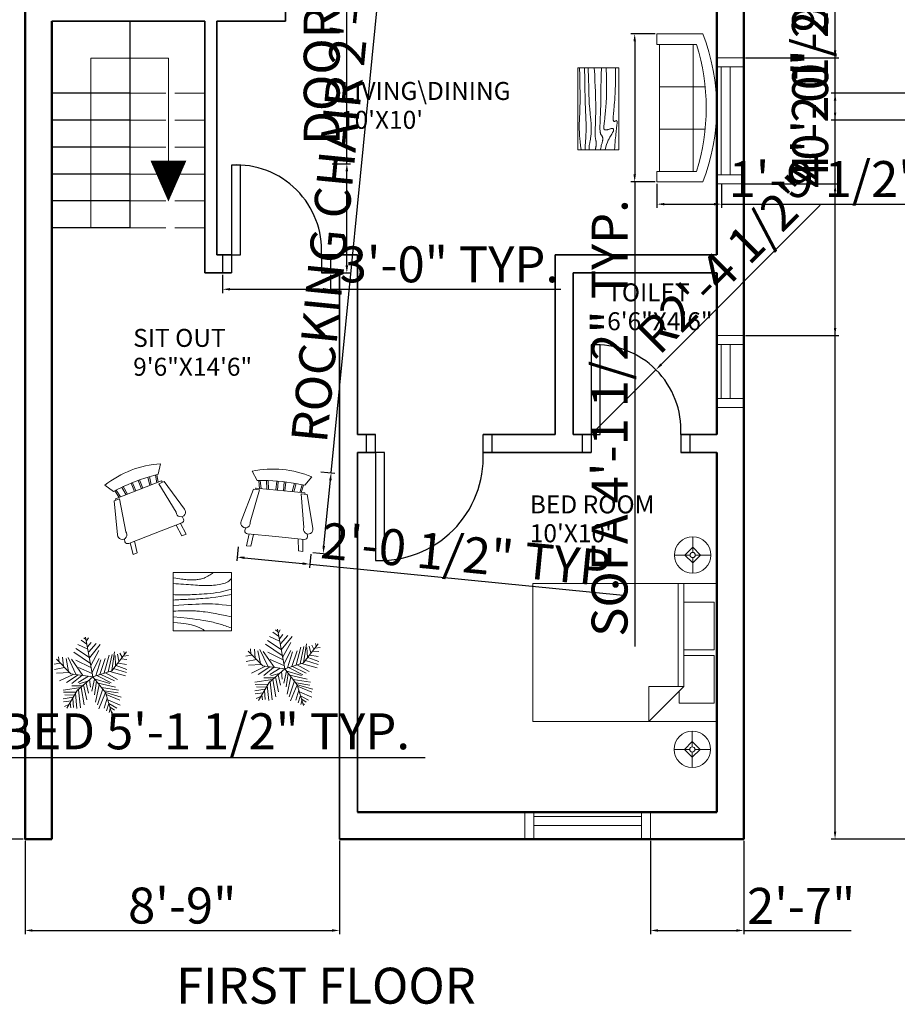
# Model space of a CAD drawing. Units: inches. Extents: x 2296 to 3335, y 495 to 1294.
# Tile 2 of 7: x 2659 to 2952, y 533 to 862. Entities that reach past the tile are written whole.
import ezdxf

# ---------------------------------------------------------------- set-up
doc = ezdxf.new("R2010")
doc.units = ezdxf.units.IN
doc.linetypes.add('ACAD_ISO02W100', pattern=[15, 12, -3])
for name, color, linetype, lineweight in [('A-ANNO-DIMS', 2, 'Continuous', 18), ('A-ANNO-SYMB', 7, 'Continuous', 18), ('A-ANNO-TEXT', 7, 'Continuous', 35), ('A-AREA-IDEN', 7, 'Continuous', 18), ('A-FLOR-STRS', 7, 'Continuous', 25), ('A-FLOR-STRS-OVHD', 7, 'ACAD_ISO02W100', 18), ('DOORS', 1, 'Continuous', 25), ('E-LITE', 2, 'Continuous', 18), ('FURNITURE', 2, 'Continuous', 18), ('INNER WALL', 6, 'Continuous', 35), ('L-PLNT', 3, 'Continuous', 13), ('OUTER WALL', 5, 'Continuous', 50), ('VENTILATOR', 4, 'Continuous', 18), ('WINDOWS', 3, 'Continuous', 18)]:
    doc.layers.add(name, color=color, linetype=linetype, lineweight=lineweight)
doc.styles.get("Standard").update_dxf_attribs({"font": 'arial.ttf'})
doc.dimstyles.new('ISO-25', dxfattribs={"dimtxt": 12, "dimasz": 2.5, "dimexe": 1.25, "dimexo": 0.625, "dimtad": 1, "dimdec": 1, "dimlunit": 3, "dimtxsty": 'Standard', "dimcen": 2.5, "dimadec": 0, "dimazin": 0, "dimtfac": 1, "dimtdec": 1, "dimtmove": 0, "dimatfit": 3, "dimfxl": 1, "dimarcsym": 0})

# ---------------------------------------------------------------- blocks, each defined once
blk = doc.blocks.new('Chair - Rocking')
for p, q in [((-8, -4.5), (-10, -1.5)), ((8, -4.5), (10, -1.5)), ((-7.5, -4.5), (-7, -7)), ((-6.5, -7), (-7.02225, -4.43)), ((-4.5, -7), (-4.96674, -4.19951)), ((-4, -7), (-4.40532, -4.16272)), ((-1.5, -4.05012), (-1.5, -7)), ((-1, -7), (-1, -4.05012)), ((1, -7), (1, -4.04655)), ((1.5, -4.05012), (1.5, -7)), ((4, -7), (4.40187, -4.18694)), ((4.5, -7), (4.96761, -4.19437)), ((6.5, -7), (7, -4.4057)), ((7.5, -4.5), (7, -7)), ((-9, -7.5), (-12, -18.49999)), ((-7, -7.5), (-9, -7.5)), ((-9, -18.49999), (-7, -7.5)), ((-8.23428, -6.99939), (-8.3093, -7.47958)), ((-8.23041, -7), (8.23915, -7)), ((7, -7.5), (9, -7.5)), ((9, -18.49999), (7, -7.5)), ((8.31071, -7.48854), (8.23449, -7.00073)), ((9, -7.5), (12, -18.49999)), ((-10.36644, -20.64523), (-10.5, -21.49999)), ((-9, -22.49999), (-9.5, -26.49999)), ((0, -22.49999), (-9.5, -22.49999)), ((-8, -26.49999), (-7.5, -22.49999)), ((0, -22.49999), (9.5, -22.49999)), ((8, -26.49999), (7.5, -22.49999)), ((9, -22.49999), (9.5, -26.49999)), ((10.5, -21.49999), (10.3575, -20.58798)), ((-9.5, -26.49999), (-8, -26.49999)), ((9.5, -26.49999), (8, -26.49999))]:
    blk.add_line(p, q)
for centre, radius, start, end in [((0, -34.08333), 34.08333, 72.93847, 107.0615), ((0, -68.25004), 64.25, 93.92211, 97.15267), ((0, -68.25004), 64.25, 82.84733, 93.92211), ((-10.5, -18.99999), 1.58114, 161.5651, 18.43495), ((10.5, -18.99999), 1.58114, 161.5651, 18.43495), ((-9.5, -21.49999), 1, 180, 270), ((9.5, -21.49999), 1, 270, 0)]:
    blk.add_arc(centre, radius, start, end)
blk = doc.blocks.new('Table - Square Woodgrain 42 x 42 in.')
blk.add_line((0, -42), (42, -42))
for points in [[(0, -4), (1.704, -4.2172), (3.2358, -4.4188), (4.615, -4.604), (5.8615, -4.7721), (6.9951, -4.9224), (8.0357, -5.0541), (9.0031, -5.1667), (9.9171, -5.2594), (10.7951, -5.3316), (11.6445, -5.3836), (12.4702, -5.4157), (13.277, -5.4283), (14.0698, -5.4217), (14.8535, -5.3964), (15.6331, -5.3526), (16.4133, -5.2908), (17.1986, -5.2103), (17.9913, -5.1062), (18.793, -4.9727), (19.6056, -4.8038), (20.4307, -4.5937), (21.2701, -4.3365), (22.1256, -4.0262), (22.9989, -3.6571), (23.888, -3.2272), (24.7756, -2.7516), (25.6408, -2.2491), (26.4624, -1.7387), (27.2195, -1.2395), (27.891, -0.7703), (28.456, -0.3501), (28.8934, 0.002)], [(0, -42), (0, 0), (42, 0), (42, -42)], [(0, -8), (1.8203, -8.1001), (3.6741, -8.2149), (5.5411, -8.3408), (7.4011, -8.4741), (9.2339, -8.6112), (11.0193, -8.7484), (12.7371, -8.8821), (14.3671, -9.0086), (15.8954, -9.1246), (17.3337, -9.2278), (18.6997, -9.3159), (20.0116, -9.387), (21.2871, -9.4389), (22.5442, -9.4696), (23.8008, -9.477), (25.0749, -9.459), (26.3791, -9.4137), (27.7049, -9.3403), (29.0383, -9.2382), (30.3655, -9.1068), (31.6728, -8.9455), (32.9461, -8.7535), (34.1717, -8.5304), (35.3358, -8.2756), (36.4268, -7.9863), (37.443, -7.6521), (38.3849, -7.2603), (39.253, -6.7986), (40.048, -6.2542), (40.7705, -5.6147), (41.421, -4.8674), (42, -4)], [(42, -12), (39.1784, -12.8621), (36.4519, -13.5654), (33.8246, -14.1294), (31.3004, -14.5731), (28.8832, -14.9161), (26.577, -15.1775), (24.3858, -15.3768), (22.3136, -15.5332), (20.3622, -15.6632), (18.5254, -15.7718), (16.7947, -15.8612), (15.1618, -15.9338), (13.6183, -15.9916), (12.1558, -16.0369), (10.7659, -16.0718), (9.4403, -16.0987), (8.1703, -16.1191), (6.9461, -16.1325), (5.7577, -16.1377), (4.595, -16.1335), (3.4479, -16.1188), (2.3064, -16.0924), (1.1604, -16.0532), (0, -16)], [(42, -16), (37.6529, -16.7365), (33.8802, -17.329), (30.6179, -17.7961), (27.8015, -18.1561), (25.3668, -18.4275), (23.2497, -18.6288), (21.3859, -18.7785), (19.7111, -18.8949), (18.1693, -18.9939), (16.7375, -19.0795), (15.401, -19.1534), (14.1449, -19.217), (12.9544, -19.2717), (11.8148, -19.3191), (10.7113, -19.3606), (9.6291, -19.3976), (8.5534, -19.4323), (7.47, -19.4689), (6.3643, -19.5122), (5.222, -19.5672), (4.0288, -19.6386), (2.7703, -19.7313), (1.4321, -19.8501), (0, -20)], [(0, -24), (3.9243, -23.6805), (7.4766, -23.4138), (10.6891, -23.1954), (13.5943, -23.0205), (16.2247, -22.8847), (18.6125, -22.7832), (20.7903, -22.7116), (22.7903, -22.6651), (24.6563, -22.642), (26.4764, -22.6507), (28.35, -22.7024), (30.3766, -22.8084), (32.6555, -22.98), (35.2861, -23.2283), (38.3678, -23.5645), (42, -24)], [(42, -32), (37.392, -31.017), (33.4585, -30.2231), (30.1291, -29.5949), (27.3334, -29.109), (25.0009, -28.742), (23.0612, -28.4707), (21.4439, -28.2716), (20.0786, -28.1215), (18.8998, -28.0002), (17.8609, -27.9014), (16.9206, -27.8219), (16.0371, -27.7588), (15.1691, -27.709), (14.2748, -27.6693), (13.3128, -27.6368), (12.2415, -27.6083), (11.0295, -27.5824), (9.6867, -27.5643), (8.233, -27.5608), (6.6884, -27.5787), (5.0728, -27.6248), (3.4062, -27.7058), (1.7086, -27.8286), (0, -28)], [(0, -32), (5.4026, -32.5358), (9.9494, -33.019), (13.7424, -33.4553), (16.8834, -33.8505), (19.4743, -34.2106), (21.6171, -34.5413), (23.4136, -34.8486), (24.9657, -35.1382), (26.3614, -35.4156), (27.6332, -35.6841), (28.7995, -35.9467), (29.8788, -36.2064), (30.8897, -36.4661), (31.8507, -36.7288), (32.7802, -36.9973), (33.6968, -37.2747), (34.6175, -37.5635), (35.5531, -37.8651), (36.5128, -38.1805), (37.506, -38.5108), (38.5421, -38.8568), (39.6302, -39.2197), (40.7797, -39.6004), (42, -40)], [(0, -36), (3.0098, -36.2857), (5.5354, -36.5643), (7.6368, -36.8359), (9.374, -37.1009), (10.807, -37.3597), (11.9957, -37.6126), (13.0002, -37.8599), (13.8804, -38.102), (14.6874, -38.3393), (15.4365, -38.5729), (16.1338, -38.8041), (16.7858, -39.0341), (17.3987, -39.264), (17.9787, -39.4952), (18.5322, -39.7288), (19.0655, -39.9662), (19.5832, -40.2081), (20.0842, -40.4544), (20.5657, -40.7046), (21.0249, -40.9581), (21.459, -41.2144), (21.8653, -41.4731), (22.2409, -41.7335), (22.5831, -41.9951)]]:
    blk.add_lwpolyline(points)
blk = doc.blocks.new('Sofa - Roundback 7 ft.')
for p, q in [((-12.00002, -32.4421), (-12.00003, -6.5971)), ((11.99997, -32.4421), (11.99998, -6.5971)), ((-36.000027, -34), (-36.000027, -11.4696)), ((-35.999844, -13.3819), (35.9998, -13.3819)), ((35.99998, -34), (35.99998, -11.4696)), ((-36.000027, -32.4421), (35.99998, -32.4421))]:
    blk.add_line(p, q)
for points in [[(-36.000027, -34), (-42.000027, -34), (-42.000027, -8)], [(41.99998, -8), (41.99998, -34), (35.99998, -34)]]:
    blk.add_lwpolyline(points)
for centre, radius, start, end in [((0, -114.25), 114.25, 68.43141, 111.5686), ((-0.00001, -127.1968), 121.1968, 72.72033, 107.2797)]:
    blk.add_arc(centre, radius, start, end)
blk = doc.blocks.new('Table - Rectangular Woodgrain 60 x 30 in.')
for p, q in [((0, 0), (0, -30)), ((60, 0), (0, 0)), ((60, -30), (60, 0)), ((0, -30), (60, -30))]:
    blk.add_line(p, q)
for points in [[(0, -2.4), (4.8155, -2.418), (9.0302, -2.4688), (12.709, -2.5477), (15.9167, -2.65), (18.7181, -2.7711), (21.1781, -2.9063), (23.3616, -3.0508), (25.3333, -3.2), (27.1477, -3.3495), (28.8172, -3.4958), (30.3437, -3.636), (31.7291, -3.7667), (32.9756, -3.8849), (34.0849, -3.9875), (35.059, -4.0714), (35.9, -4.1334), (36.6114, -4.1711), (37.2041, -4.1854), (37.6906, -4.1779), (38.0833, -4.15), (38.3948, -4.1034), (38.6375, -4.0396), (38.8239, -3.9602), (38.9666, -3.8667), (39.0764, -3.7608), (39.1573, -3.6448), (39.2116, -3.521), (39.2416, -3.3917), (39.2498, -3.2593), (39.2385, -3.1261), (39.21, -2.9944), (39.1666, -2.8667), (39.111, -2.7447), (39.0468, -2.6281), (38.978, -2.5163), (38.9083, -2.4083), (38.8418, -2.3035), (38.7823, -2.201), (38.7337, -2.1001), (38.7, -2), (38.6844, -1.9003), (38.6875, -1.8021), (38.7094, -1.707), (38.75, -1.6167), (38.8094, -1.5326), (38.8875, -1.4563), (38.9844, -1.3893), (39.1, -1.3333), (39.2351, -1.2896), (39.3937, -1.2583), (39.5804, -1.2396), (39.8, -1.2333), (40.057, -1.2396), (40.3562, -1.2583), (40.7023, -1.2896), (41.1, -1.3333), (41.5547, -1.3895), (42.0755, -1.4573), (42.6721, -1.5361), (43.3542, -1.625), (44.1316, -1.7233), (45.014, -1.8302), (46.0114, -1.9449), (47.1333, -2.0667), (48.3862, -2.1947), (49.7625, -2.3281), (51.2513, -2.4663), (52.8416, -2.6083), (54.5226, -2.7535), (56.2833, -2.9011), (58.1127, -3.0501), (60, -3.2)], [(0, -9.2), (6.5759, -9.0858), (11.9385, -9.0365), (16.2527, -9.0418), (19.6833, -9.0917), (22.3952, -9.1759), (24.5531, -9.2844), (26.322, -9.4069), (27.8666, -9.5333), (29.3241, -9.6553), (30.7203, -9.7719), (32.0532, -9.8837), (33.3208, -9.9917), (34.5213, -10.0965), (35.6526, -10.199), (36.7128, -10.2999), (37.7, -10.4), (38.6129, -10.4996), (39.4531, -10.5969), (40.223, -10.6895), (40.925, -10.775), (41.5613, -10.8512), (42.1344, -10.9156), (42.6465, -10.966), (43.1, -11), (43.4976, -11.0158), (43.8437, -11.0136), (44.143, -10.9942), (44.4, -10.9583), (44.6195, -10.9069), (44.8062, -10.8406), (44.9648, -10.7603), (45.1, -10.6667), (45.2155, -10.5598), (45.3114, -10.4365), (45.3871, -10.2929), (45.4416, -10.125), (45.4743, -9.929), (45.4844, -9.7011), (45.4709, -9.4371), (45.4333, -9.1333), (45.3716, -8.7883), (45.2896, -8.4104), (45.1919, -8.0107), (45.0833, -7.6), (44.9685, -7.1893), (44.8521, -6.7896), (44.7388, -6.4117), (44.6333, -6.0667), (44.54, -5.7628), (44.4614, -5.4979), (44.4001, -5.2675), (44.3583, -5.0667), (44.3384, -4.8909), (44.3427, -4.7354), (44.3736, -4.5956), (44.4333, -4.4667), (44.5236, -4.3453), (44.6427, -4.2333), (44.7884, -4.1339), (44.9583, -4.05), (45.1501, -3.9849), (45.3614, -3.9417), (45.59, -3.9234), (45.8333, -3.9333), (46.0915, -3.9749), (46.3734, -4.0531), (46.6906, -4.1736), (47.0542, -4.3417), (47.4756, -4.5629), (47.9661, -4.8427), (48.5372, -5.1866), (49.2, -5.6), (49.9676, -6.0844), (50.8594, -6.625), (51.8965, -7.2031), (53.1, -7.8), (54.491, -8.3969), (56.0906, -8.975), (57.9199, -9.5156), (60, -10)], [(0, -12.8), (5.1847, -12.9322), (9.6213, -13.0323), (13.3963, -13.1059), (16.5958, -13.1583), (19.3063, -13.1952), (21.614, -13.2219), (23.6054, -13.2439), (25.3666, -13.2667), (26.9728, -13.2947), (28.4531, -13.3281), (29.8256, -13.3663), (31.1083, -13.4083), (32.3191, -13.4535), (33.476, -13.501), (34.597, -13.5501), (35.7, -13.6), (36.7984, -13.6497), (37.8875, -13.6979), (38.9578, -13.743), (40, -13.7833), (41.0047, -13.8174), (41.9625, -13.8438), (42.864, -13.8607), (43.7, -13.8667), (44.4631, -13.8604), (45.1552, -13.8417), (45.7801, -13.8104), (46.3416, -13.7667), (46.8439, -13.7104), (47.2906, -13.6417), (47.6858, -13.5604), (48.0333, -13.4667), (48.3375, -13.3608), (48.6042, -13.2448), (48.8396, -13.121), (49.05, -12.9917), (49.2417, -12.8593), (49.4208, -12.7261), (49.5937, -12.5944), (49.7667, -12.4667), (49.9452, -12.3451), (50.1323, -12.2313), (50.3303, -12.1268), (50.5416, -12.0333), (50.7686, -11.9524), (51.0135, -11.8854), (51.2788, -11.8341), (51.5666, -11.8), (51.8785, -11.7843), (52.2116, -11.7865), (52.562, -11.8059), (52.926, -11.8417), (53.2998, -11.8931), (53.6795, -11.9594), (54.0614, -12.0397), (54.4416, -12.1333), (54.8223, -12.2401), (55.2293, -12.3625), (55.6942, -12.5037), (56.2489, -12.6667), (56.9251, -12.8547), (57.7545, -13.0708), (58.7689, -13.3182), (60, -13.6)], [(0, -18), (5.124, -17.7273), (9.6609, -17.5057), (13.6705, -17.3303), (17.2125, -17.1958), (20.3467, -17.0973), (23.1328, -17.0297), (25.6307, -16.9878), (27.9, -16.9667), (29.9928, -16.9617), (31.9302, -16.9703), (33.7254, -16.9907), (35.3917, -17.0208), (36.9423, -17.0588), (38.3906, -17.1026), (39.7499, -17.1503), (41.0333, -17.2), (42.2519, -17.2496), (43.4073, -17.2969), (44.4986, -17.3395), (45.525, -17.375), (46.4858, -17.4012), (47.3802, -17.4156), (48.2074, -17.416), (48.9667, -17.4), (49.6583, -17.3662), (50.2872, -17.3167), (50.8595, -17.2547), (51.3812, -17.1833), (51.8584, -17.1057), (52.2971, -17.025), (52.7034, -16.9443), (53.0833, -16.8667), (53.443, -16.7951), (53.789, -16.7313), (54.128, -16.6768), (54.4666, -16.6334), (54.8115, -16.6024), (55.1693, -16.5854), (55.5465, -16.5841), (55.95, -16.6), (56.3828, -16.6337), (56.8346, -16.6823), (57.2915, -16.7418), (57.7396, -16.8084), (58.165, -16.878), (58.5539, -16.9469), (58.8924, -17.0111), (59.1666, -17.0667), (59.3679, -17.1107), (59.5078, -17.1438), (59.6032, -17.1675), (59.6708, -17.1833), (59.7275, -17.193), (59.7901, -17.1979), (59.8753, -17.1998), (60, -17.2)], [(0, -22.4), (8.0098, -22.2501), (14.4094, -22.1011), (19.4168, -21.9535), (23.25, -21.8083), (26.1269, -21.6663), (28.2656, -21.5281), (29.884, -21.3947), (31.2, -21.2667), (32.3967, -21.1448), (33.5172, -21.0292), (34.5697, -20.9198), (35.5625, -20.8167), (36.5037, -20.7198), (37.4015, -20.6292), (38.2642, -20.5448), (39.1, -20.4667), (39.9164, -20.3951), (40.7187, -20.3313), (41.5117, -20.2768), (42.3, -20.2333), (43.0883, -20.2024), (43.8812, -20.1854), (44.6836, -20.1841), (45.5, -20.2), (46.3328, -20.234), (47.1747, -20.2844), (48.0163, -20.3488), (48.8479, -20.425), (49.66, -20.5106), (50.4429, -20.6031), (51.1872, -20.7004), (51.8833, -20.8), (52.5246, -20.8999), (53.1166, -20.9995), (53.6681, -21.0983), (54.1875, -21.1958), (54.6834, -21.2919), (55.1646, -21.3859), (55.6394, -21.4777), (56.1167, -21.5667), (56.6028, -21.6515), (57.0961, -21.7266), (57.5929, -21.7852), (58.0896, -21.8208), (58.5823, -21.8268), (59.0674, -21.7964), (59.5412, -21.723), (60, -21.6)], [(0, -25.2), (8.6355, -25.0504), (15.7026, -24.9031), (21.4049, -24.7606), (25.9458, -24.625), (29.529, -24.4988), (32.3578, -24.3844), (34.6359, -24.284), (36.5667, -24.2), (38.3213, -24.1341), (39.9417, -24.0854), (41.437, -24.0523), (42.8167, -24.0333), (44.0901, -24.0268), (45.2667, -24.0313), (46.3557, -24.0451), (47.3667, -24.0667), (48.309, -24.0947), (49.1928, -24.1287), (50.0284, -24.168), (50.826, -24.2125), (51.5959, -24.2617), (52.3483, -24.3151), (53.0935, -24.3725), (53.8417, -24.4334), (54.6009, -24.497), (55.3699, -24.561), (56.1454, -24.6226), (56.9239, -24.6792), (57.7021, -24.7279), (58.4764, -24.7662), (59.2435, -24.7911), (60, -24.8)], [(0, -28.8), (5.6867, -28.6681), (10.45, -28.5698), (14.407, -28.5012), (17.675, -28.4584), (20.3711, -28.4374), (22.6125, -28.4344), (24.5164, -28.4455), (26.2, -28.4667), (27.762, -28.4947), (29.2276, -28.5281), (30.6033, -28.5663), (31.8958, -28.6084), (33.1118, -28.6535), (34.2578, -28.7011), (35.3405, -28.7501), (36.3666, -28.8), (37.3443, -28.8497), (38.288, -28.8974), (39.2137, -28.9412), (40.1375, -28.9792), (41.0753, -29.0093), (42.0432, -29.0297), (43.0572, -29.0384), (44.1333, -29.0333), (45.2936, -29.0114), (46.5843, -28.9641), (48.0579, -28.8816), (49.7666, -28.7542), (51.7629, -28.5721), (54.0989, -28.3255), (56.8272, -28.0048), (60, -27.6)]]:
    blk.add_lwpolyline(points)
blk = doc.blocks.new('Bed - Queen')
for p, q in [((0, -80.00003), (0, 0)), ((0, 0), (59.99999, 0)), ((59.99999, 0), (59.99999, -80.00003)), ((7.99999, -1.2), (28.79998, -1.2)), ((7.99999, -14.4), (7.99999, -1.2)), ((28.79998, -1.2), (28.79998, -14.4)), ((31.19999, -1.2), (51.99999, -1.2)), ((31.19999, -14.4), (31.19999, -1.2)), ((51.99999, -1.2), (51.99999, -16.4)), ((0, -14.4), (44.8, -14.4)), ((44.8, -16.8), (0, -16.8)), ((59.99999, -29.6), (44.8, -14.4)), ((44.8, -14.4), (44.8, -29.6)), ((51.99999, -16.4), (46.79936, -16.4)), ((44.8, -29.6), (59.99999, -29.6)), ((59.99999, -80.00003), (0, -80.00003))]:
    blk.add_line(p, q)
blk = doc.blocks.new('Lamp - Table')
for p, q in [((0, 7), (0, 1)), ((-1, 0), (-7, 0)), ((0, 3), (-3, 0)), ((-3, 0), (0, -3)), ((3, 0), (0, 3)), ((0, -3), (3, 0)), ((1, 0), (7, 0)), ((0, -1), (0, -7))]:
    blk.add_line(p, q)
for radius in [7, 1]:
    blk.add_circle((0, 0), radius)
blk = doc.blocks.new('*U15')
for p, q in [((0, 0), (-10.5, 57)), ((-7.288, 39.707), (-21.778, 46.673)), ((-8.737, 47.138), (-17.069, 52.711)), ((-10.186, 53.64), (-13.084, 55.962)), ((-9.099, 51.782), (-6.563, 55.962)), ((-7.65, 43.423), (-2.578, 49.46)), ((-5.839, 35.992), (4.667, 48.067)), ((-5.114, 27.632), (10.463, 46.673)), ((-48.585, 21.131), (-49.309, 29.026)), ((-43.513, 28.561), (-42.427, 15.558)), ((-3.665, 19.273), (-27.574, 35.527)), ((-5.114, 28.097), (-24.676, 40.636)), ((-2.941, 16.486), (8.652, 37.85)), ((16.259, 5.805), (23.142, 31.348)), ((22.055, 7.198), (27.489, 32.277)), ((27, 9), (48, 36)), ((27.127, 9.056), (31.112, 35.992)), ((31.836, 30.883), (32.561, 16.486)), ((35.096, 32.741), (37.27, 22.524)), ((38.719, 34.134), (41.979, 28.561)), ((43.791, 29.954), (51.036, 30.883)), ((44.153, 36.456), (45.239, 32.741)), ((-47.498, 19.737), (-55.83, 18.344)), ((-31.5, 4.5), (-52.5, 25.5)), ((-38.442, 26.239), (-34.819, 7.663)), ((-35.544, 28.097), (-24.314, 3.947)), ((-14.533, 2.09), (-30.834, 25.31)), ((-24.314, 23.917), (-2.941, 13.7)), ((-1.129, 6.734), (9.014, 26.704)), ((3.942, 1.625), (11.187, 24.381)), ((10.101, 3.483), (17.708, 26.239)), ((33.285, 16.486), (48.862, 10.913)), ((36.183, 19.737), (48.137, 17.88)), ((40.53, 25.775), (48.862, 24.846)), ((-40.615, 13.7), (-55.105, 10.913)), ((-33.37, 6.269), (-52.207, 5.34)), ((-28.299, 3.483), (-47.86, -5.805)), ((-21.416, 3.018), (-38.079, -8.128)), ((0, 0), (-31.5, 4.5)), ((-15.982, 2.09), (-30.11, -9.521)), ((0, 0), (-22.5, -19.5)), ((-6.563, 1.161), (-21.416, -8.128)), ((-20.691, 13.7), (-1.129, 4.876)), ((0, 0), (27, 9)), ((0, 0), (18, -22.5)), ((6.478, 1.625), (26.04, -8.592)), ((11.187, 3.483), (30.749, -5.805)), ((18.07, 5.805), (35.096, -3.483)), ((24.229, 7.663), (46.688, 1.625)), ((29.662, 12.307), (48.137, 6.269)), ((-15.257, -12.772), (-30.11, -12.772)), ((-6.563, -5.805), (-19.967, -9.985)), ((-13.446, -11.378), (-8.737, -32.741)), ((-9.461, -8.592), (-6.201, -23.453)), ((-4.752, -3.483), (-3.665, -14.629)), ((2.493, -3.019), (-1.491, -20.202)), ((1.769, -2.555), (24.229, -9.521)), ((5.029, -6.27), (2.131, -25.775)), ((9.014, -11.378), (3.58, -35.992)), ((7.565, -9.056), (32.198, -14.629)), ((-17.431, -15.094), (-42.789, -18.809)), ((-24.314, -21.596), (-42.427, -22.06)), ((-26.849, -26.24), (-40.253, -25.775)), ((-22.5, -19.5), (-37.5, -45)), ((-25.038, -23.918), (-22.865, -45.281)), ((-20.691, -18.345), (-17.793, -44.352)), ((-17.069, -15.094), (-12.721, -40.172)), ((14.085, -16.951), (6.478, -40.172)), ((18.07, -22.524), (8.289, -45.745)), ((12.274, -15.094), (36.907, -18.809)), ((16.259, -19.738), (36.183, -22.989)), ((18, -22.5), (27, -52.5)), ((18.433, -22.524), (40.53, -29.026)), ((19.157, -25.311), (38.719, -33.206)), ((-28.299, -29.026), (-42.789, -31.348)), ((-30.834, -34.135), (-42.427, -35.528)), ((-34.457, -39.708), (-40.978, -42.494)), ((-32.646, -36.921), (-31.921, -44.352)), ((-29.023, -30.884), (-27.936, -43.887)), ((20.244, -30.419), (15.897, -44.816)), ((22.78, -37.85), (19.519, -48.532)), ((21.331, -32.741), (39.081, -40.636)), ((22.78, -38.314), (34.372, -44.816)), ((24.591, -45.745), (23.142, -50.854)), ((24.591, -43.423), (30.749, -47.603)), ((26.764, -49.925), (28.213, -50.854))]:
    blk.add_line(p, q)
blk = doc.blocks.new('DOOR-SINGLE-30IN')
for p, q in [((-3, 0), (-3, -6)), ((0, 0), (0, -6)), ((30, 0), (30, -6)), ((33, 0), (33, -6))]:
    blk.add_line(p, q)
blk.add_lwpolyline([(0, 0), (3, 0), (3, 30), (0, 30)], close=True)
blk.add_arc((1.5, 1.5), 28.54, 356.9872, 93.0128)
blk = doc.blocks.new('DOOR-SINGLE-36IN')
for p, q in [((0, 39), (-6, 39)), ((0, 36), (-6, 36)), ((0, 0), (-6, 0)), ((0, -3), (-6, -3))]:
    blk.add_line(p, q)
blk.add_lwpolyline([(0, 0), (36, 0), (36, 3), (0, 3)], close=True)
blk.add_arc((1.5, 1.5), 34.53, 357.5104, 92.4896)
blk = doc.blocks.new('WIN-36IN')
for p, q in [((0, 42), (9, 42)), ((0, 39), (9, 39)), ((1.5, 3), (1.5, 39)), ((4.5, 3), (4.5, 39)), ((9, 3), (0, 3)), ((9, 0), (0, 0))]:
    blk.add_line(p, q)
blk = doc.blocks.new('VENT-18IN')
for p, q in [((0, 24), (9, 24)), ((0, 21), (9, 21)), ((4.5, 21), (4.5, 3)), ((7.5, 21), (7.5, 3)), ((9, 3), (0, 3)), ((9, 0), (0, 0))]:
    blk.add_line(p, q)
blk = doc.blocks.new('*D27')
at = {"layer": 'A-ANNO-DIMS', "color": 0, "lineweight": -2, "transparency": 16777216}
for p, q in [((2524.66, 623.83), (2524.66, 613.99)), ((2586.06, 623.83), (2586.06, 613.99)), ((2527.16, 615.24), (2583.56, 615.24)), ((2586.06, 615.24), (2794.3, 615.24))]:
    blk.add_line(p, q, dxfattribs=at)
at = {"layer": 'A-ANNO-DIMS', "color": 0, "transparency": 16777216}
for points in [[(2527.16, 615.66), (2527.16, 614.82), (2524.66, 615.24)], [(2583.56, 615.66), (2583.56, 614.82), (2586.06, 615.24)]]:
    blk.add_solid(points, dxfattribs=at)
at = {"layer": 'Defpoints', "color": 0, "transparency": 16777216}
for p in [(2524.66, 624.45), (2586.06, 624.45), (2586.06, 615.24)]:
    blk.add_point(p, dxfattribs=at)
at = {"layer": 'A-ANNO-DIMS', "color": 0, "transparency": 16777216, "insert": (2691.43, 622.44), "char_height": 12, "attachment_point": 5}
blk.add_mtext('QUEEN BED 5\'-1 1/2" TYP.', dxfattribs=at)
blk = doc.blocks.new('*D37')
at = {"layer": 'A-ANNO-DIMS', "color": 0, "lineweight": -2, "transparency": 16777216}
for p, q in [((2768.12, 813.44), (2768.12, 998.74)), ((2763.28, 813.44), (2769.37, 813.44)), ((2768.12, 779.52), (2768.12, 810.94)), ((2763.28, 777.02), (2769.37, 777.02))]:
    blk.add_line(p, q, dxfattribs=at)
at = {"layer": 'A-ANNO-DIMS', "color": 0, "transparency": 16777216}
for points in [[(2767.7, 810.94), (2768.54, 810.94), (2768.12, 813.44)], [(2767.7, 779.52), (2768.54, 779.52), (2768.12, 777.02)]]:
    blk.add_solid(points, dxfattribs=at)
at = {"layer": 'Defpoints', "color": 0, "transparency": 16777216}
for p in [(2762.66, 813.44), (2768.12, 813.44), (2762.66, 777.02)]:
    blk.add_point(p, dxfattribs=at)
at = {"layer": 'A-ANNO-DIMS', "color": 0, "transparency": 16777216, "insert": (2761.28, 907.34), "char_height": 12, "attachment_point": 5, "rotation": 90}
blk.add_mtext('DOOR D1 3\'-0 1/2" TYP.', dxfattribs=at)
blk = doc.blocks.new('*D38')
at = {"layer": 'A-ANNO-DIMS', "color": 0, "lineweight": -2, "transparency": 16777216}
for p, q in [((2726.66, 776.39), (2726.66, 770.3)), ((2762.66, 776.39), (2762.66, 770.3)), ((2729.16, 771.55), (2760.16, 771.55)), ((2762.66, 771.55), (2839.55, 771.55))]:
    blk.add_line(p, q, dxfattribs=at)
at = {"layer": 'A-ANNO-DIMS', "color": 0, "transparency": 16777216}
for points in [[(2729.16, 771.97), (2729.16, 771.14), (2726.66, 771.55)], [(2760.16, 771.97), (2760.16, 771.14), (2762.66, 771.55)]]:
    blk.add_solid(points, dxfattribs=at)
at = {"layer": 'Defpoints', "color": 0, "transparency": 16777216}
for p in [(2726.66, 777.02), (2762.66, 777.02), (2762.66, 771.55)]:
    blk.add_point(p, dxfattribs=at)
at = {"layer": 'A-ANNO-DIMS', "color": 0, "transparency": 16777216, "insert": (2802.35, 778.31), "char_height": 12, "attachment_point": 5}
blk.add_mtext('3\'-0" TYP.', dxfattribs=at)
blk = doc.blocks.new('*D43')
at = {"layer": 'A-ANNO-DIMS', "color": 0, "lineweight": -2, "transparency": 16777216}
for p, q in [((2871.03, 856.78), (2862.99, 856.78)), ((2864.24, 854.28), (2864.24, 809.87)), ((2871.03, 807.37), (2862.99, 807.37)), ((2864.24, 807.37), (2864.24, 652.27))]:
    blk.add_line(p, q, dxfattribs=at)
at = {"layer": 'A-ANNO-DIMS', "color": 0, "transparency": 16777216}
for points in [[(2863.83, 854.28), (2864.66, 854.28), (2864.24, 856.78)], [(2863.83, 809.87), (2864.66, 809.87), (2864.24, 807.37)]]:
    blk.add_solid(points, dxfattribs=at)
at = {"layer": 'Defpoints', "color": 0, "transparency": 16777216}
for p in [(2871.66, 856.78), (2864.24, 807.37), (2871.66, 807.37)]:
    blk.add_point(p, dxfattribs=at)
at = {"layer": 'A-ANNO-DIMS', "color": 0, "transparency": 16777216, "insert": (2857.41, 728.57), "char_height": 12, "attachment_point": 5, "rotation": 90}
blk.add_mtext('SOFA 4\'-1 1/2" TYP.', dxfattribs=at)
blk = doc.blocks.new('*D44')
at = {"layer": 'A-ANNO-DIMS', "color": 0, "lineweight": -2, "transparency": 16777216}
for p, q in [((2871.66, 806.74), (2871.66, 798.71)), ((2893.23, 806.74), (2893.23, 798.71)), ((2874.16, 799.96), (2890.73, 799.96)), ((2893.23, 799.96), (2996.95, 799.96))]:
    blk.add_line(p, q, dxfattribs=at)
at = {"layer": 'A-ANNO-DIMS', "color": 0, "transparency": 16777216}
for points in [[(2874.16, 800.37), (2874.16, 799.54), (2871.66, 799.96)], [(2890.73, 800.37), (2890.73, 799.54), (2893.23, 799.96)]]:
    blk.add_solid(points, dxfattribs=at)
at = {"layer": 'Defpoints', "color": 0, "transparency": 16777216}
for p in [(2871.66, 807.37), (2893.23, 807.37), (2893.23, 799.96)]:
    blk.add_point(p, dxfattribs=at)
at = {"layer": 'A-ANNO-DIMS', "color": 0, "transparency": 16777216, "insert": (2946.34, 806.78), "char_height": 12, "attachment_point": 5}
blk.add_mtext('1\'-9 1/2" TYP.', dxfattribs=at)
blk = doc.blocks.new('*D47')
at = {"layer": 'A-ANNO-DIMS', "color": 0, "lineweight": -2, "transparency": 16777216}
for p, q in [((2762.87, 710.27), (2784.09, 925.21)), ((2759.46, 710.6), (2764.11, 710.14)), ((2760.46, 685.88), (2762.62, 707.78)), ((2756.81, 683.73), (2761.46, 683.27))]:
    blk.add_line(p, q, dxfattribs=at)
at = {"layer": 'A-ANNO-DIMS', "color": 0, "transparency": 16777216}
for points in [[(2762.21, 707.82), (2763.04, 707.74), (2762.87, 710.27)], [(2760.04, 685.93), (2760.87, 685.84), (2760.21, 683.4)]]:
    blk.add_solid(points, dxfattribs=at)
at = {"layer": 'Defpoints', "color": 0, "transparency": 16777216}
for p in [(2758.84, 710.66), (2762.87, 710.27), (2756.18, 683.79)]:
    blk.add_point(p, dxfattribs=at)
at = {"layer": 'A-ANNO-DIMS', "color": 0, "transparency": 16777216, "insert": (2766.79, 819.65), "char_height": 12, "attachment_point": 5, "rotation": 84.3621}
blk.add_mtext('ROCKING CHAIR 2\'-3" TYP.', dxfattribs=at)
blk = doc.blocks.new('*D48')
at = {"layer": 'A-ANNO-DIMS', "color": 0, "lineweight": -2, "transparency": 16777216}
for p, q in [((2731.81, 685.57), (2731.35, 680.92)), ((2733.96, 681.92), (2753.3, 680.01)), ((2756.12, 683.17), (2755.66, 678.52)), ((2755.79, 679.76), (2860.34, 669.44))]:
    blk.add_line(p, q, dxfattribs=at)
at = {"layer": 'A-ANNO-DIMS', "color": 0, "transparency": 16777216}
for points in [[(2734, 682.33), (2733.92, 681.5), (2731.47, 682.16)], [(2753.34, 680.42), (2753.26, 679.6), (2755.79, 679.76)]]:
    blk.add_solid(points, dxfattribs=at)
at = {"layer": 'Defpoints', "color": 0, "transparency": 16777216}
for p in [(2731.87, 686.2), (2756.18, 683.79), (2755.79, 679.76)]:
    blk.add_point(p, dxfattribs=at)
at = {"layer": 'A-ANNO-DIMS', "color": 0, "transparency": 16777216, "insert": (2809.98, 681.28), "char_height": 12, "attachment_point": 5, "rotation": 354.3621}
blk.add_mtext('2\'-0 1/2" TYP.', dxfattribs=at)
blk = doc.blocks.new('*D52')
at = {"layer": 'A-ANNO-DIMS', "color": 0, "lineweight": -2, "transparency": 16777216}
for p, q in [((2660.03, 1068.02), (2628.91, 1068.02)), ((2630.16, 590.52), (2630.16, 1065.52)), ((2660.03, 588.02), (2628.91, 588.02))]:
    blk.add_line(p, q, dxfattribs=at)
at = {"layer": 'A-ANNO-DIMS', "color": 0, "transparency": 16777216}
for points in [[(2629.74, 1065.52), (2630.57, 1065.52), (2630.16, 1068.02)], [(2629.74, 590.52), (2630.57, 590.52), (2630.16, 588.02)]]:
    blk.add_solid(points, dxfattribs=at)
at = {"layer": 'Defpoints', "color": 0, "transparency": 16777216}
for p in [(2630.16, 1068.02), (2660.66, 1068.02), (2660.66, 588.02)]:
    blk.add_point(p, dxfattribs=at)
at = {"layer": 'A-ANNO-DIMS', "color": 0, "transparency": 16777216, "insert": (2623.41, 828.02), "char_height": 12, "attachment_point": 5, "rotation": 90}
blk.add_mtext('40\'-0"', dxfattribs=at)
blk = doc.blocks.new('*D54')
at = {"layer": 'A-ANNO-DIMS', "color": 0, "lineweight": -2, "transparency": 16777216}
for p, q in [((2961.02, 1068.02), (2929.9, 1068.02)), ((2931.15, 590.52), (2931.15, 1065.52)), ((2961.02, 588.02), (2929.9, 588.02))]:
    blk.add_line(p, q, dxfattribs=at)
at = {"layer": 'A-ANNO-DIMS', "color": 0, "transparency": 16777216}
for points in [[(2930.73, 1065.52), (2931.56, 1065.52), (2931.15, 1068.02)], [(2930.73, 590.52), (2931.56, 590.52), (2931.15, 588.02)]]:
    blk.add_solid(points, dxfattribs=at)
at = {"layer": 'Defpoints', "color": 0, "transparency": 16777216}
for p in [(2931.15, 1068.02), (2961.65, 1068.02), (2961.65, 588.02)]:
    blk.add_point(p, dxfattribs=at)
at = {"layer": 'A-ANNO-DIMS', "color": 0, "transparency": 16777216, "insert": (2924.39, 828.02), "char_height": 12, "attachment_point": 5, "rotation": 90}
blk.add_mtext('40\'-0"', dxfattribs=at)
blk = doc.blocks.new('*D66')
at = {"layer": 'A-ANNO-DIMS', "color": 0, "lineweight": -2, "transparency": 16777216}
for p, q in [((2931.15, 837.02), (2931.15, 872.67)), ((2970.02, 837.02), (2929.9, 837.02)), ((2931.15, 830.52), (2931.15, 834.52)), ((2970.02, 828.02), (2929.9, 828.02))]:
    blk.add_line(p, q, dxfattribs=at)
at = {"layer": 'A-ANNO-DIMS', "color": 0, "transparency": 16777216}
for points in [[(2930.73, 834.52), (2931.56, 834.52), (2931.15, 837.02)], [(2930.73, 830.52), (2931.56, 830.52), (2931.15, 828.02)]]:
    blk.add_solid(points, dxfattribs=at)
at = {"layer": 'Defpoints', "color": 0, "transparency": 16777216}
for p in [(2931.15, 837.02), (2970.65, 837.02), (2970.65, 828.02)]:
    blk.add_point(p, dxfattribs=at)
at = {"layer": 'A-ANNO-DIMS', "color": 0, "transparency": 16777216, "insert": (2924.39, 856.09), "char_height": 12, "attachment_point": 5, "rotation": 90}
blk.add_mtext('0\'-9"', dxfattribs=at)
blk = doc.blocks.new('*D68')
at = {"layer": 'A-ANNO-DIMS', "color": 0, "lineweight": -2, "transparency": 16777216}
for p, q in [((2901.28, 948.82), (2932.41, 948.82)), ((2931.16, 851.25), (2931.16, 946.32)), ((2901.28, 848.75), (2932.41, 848.75))]:
    blk.add_line(p, q, dxfattribs=at)
at = {"layer": 'A-ANNO-DIMS', "color": 0, "transparency": 16777216}
for points in [[(2930.74, 946.32), (2931.57, 946.32), (2931.16, 948.82)], [(2930.74, 851.25), (2931.57, 851.25), (2931.16, 848.75)]]:
    blk.add_solid(points, dxfattribs=at)
at = {"layer": 'Defpoints', "color": 0, "transparency": 16777216}
for p in [(2900.66, 948.82), (2931.16, 948.82), (2900.66, 848.75)]:
    blk.add_point(p, dxfattribs=at)
at = {"layer": 'A-ANNO-DIMS', "color": 0, "transparency": 16777216, "insert": (2924.41, 898.79), "char_height": 12, "attachment_point": 5, "rotation": 90}
blk.add_mtext('8\'-4"', dxfattribs=at)
blk = doc.blocks.new('*D69')
at = {"layer": 'A-ANNO-DIMS', "color": 0, "lineweight": -2, "transparency": 16777216}
for p, q in [((2931.16, 806.75), (2931.16, 870.85)), ((2901.28, 806.75), (2932.41, 806.75)), ((2931.16, 758.61), (2931.16, 804.25)), ((2901.28, 756.11), (2932.41, 756.11))]:
    blk.add_line(p, q, dxfattribs=at)
at = {"layer": 'A-ANNO-DIMS', "color": 0, "transparency": 16777216}
for points in [[(2930.74, 804.25), (2931.57, 804.25), (2931.16, 806.75)], [(2930.74, 758.61), (2931.57, 758.61), (2931.16, 756.11)]]:
    blk.add_solid(points, dxfattribs=at)
at = {"layer": 'Defpoints', "color": 0, "transparency": 16777216}
for p in [(2900.66, 806.75), (2931.16, 806.75), (2900.66, 756.11)]:
    blk.add_point(p, dxfattribs=at)
at = {"layer": 'A-ANNO-DIMS', "color": 0, "transparency": 16777216, "insert": (2924.33, 840.05), "char_height": 12, "attachment_point": 5, "rotation": 90}
blk.add_mtext('4\'-2 1/2"', dxfattribs=at)
blk = doc.blocks.new('*D71')
at = {"layer": 'A-ANNO-DIMS', "color": 0, "lineweight": -2, "transparency": 16777216}
for p, q in [((2869.55, 587.39), (2869.55, 556.27)), ((2900.66, 587.39), (2900.66, 556.27)), ((2872.05, 557.52), (2898.16, 557.52)), ((2900.66, 557.52), (2936.51, 557.52))]:
    blk.add_line(p, q, dxfattribs=at)
at = {"layer": 'A-ANNO-DIMS', "color": 0, "transparency": 16777216}
for points in [[(2872.05, 557.93), (2872.05, 557.1), (2869.55, 557.52)], [(2898.16, 557.93), (2898.16, 557.1), (2900.66, 557.52)]]:
    blk.add_solid(points, dxfattribs=at)
at = {"layer": 'Defpoints', "color": 0, "transparency": 16777216}
for p in [(2869.55, 588.02), (2900.66, 588.02), (2900.66, 557.52)]:
    blk.add_point(p, dxfattribs=at)
at = {"layer": 'A-ANNO-DIMS', "color": 0, "transparency": 16777216, "insert": (2919.83, 564.17), "char_height": 12, "attachment_point": 5}
blk.add_mtext('2\'-7"', dxfattribs=at)
blk = doc.blocks.new('*D72')
at = {"layer": 'A-ANNO-DIMS', "color": 0, "lineweight": -2, "transparency": 16777216}
for p, q in [((2660.66, 587.39), (2660.66, 556.27)), ((2765.66, 587.39), (2765.66, 556.27)), ((2663.16, 557.52), (2763.16, 557.52))]:
    blk.add_line(p, q, dxfattribs=at)
at = {"layer": 'A-ANNO-DIMS', "color": 0, "transparency": 16777216}
for points in [[(2663.16, 557.93), (2663.16, 557.1), (2660.66, 557.52)], [(2763.16, 557.93), (2763.16, 557.1), (2765.66, 557.52)]]:
    blk.add_solid(points, dxfattribs=at)
at = {"layer": 'Defpoints', "color": 0, "transparency": 16777216}
for p in [(2660.66, 588.02), (2765.66, 588.02), (2765.66, 557.52)]:
    blk.add_point(p, dxfattribs=at)
at = {"layer": 'A-ANNO-DIMS', "color": 0, "transparency": 16777216, "insert": (2713.16, 564.27), "char_height": 12, "attachment_point": 5}
blk.add_mtext('8\'-9"', dxfattribs=at)
blk = doc.blocks.new('*D80')
at = {"layer": 'A-ANNO-DIMS', "color": 0, "lineweight": -2, "transparency": 16777216}
for p, q in [((2926.21, 799.57), (2873.11, 746.47)), ((2851.16, 724.52), (2871.34, 744.7))]:
    blk.add_line(p, q, dxfattribs=at)
at = {"layer": 'A-ANNO-DIMS', "color": 0, "transparency": 16777216}
blk.add_solid([(2872.81, 746.76), (2873.4, 746.17), (2871.34, 744.7)], dxfattribs=at)
at = {"layer": 'Defpoints', "color": 0, "transparency": 16777216}
for p in [(2871.34, 744.7), (2851.16, 724.52)]:
    blk.add_point(p, dxfattribs=at)
at = {"layer": 'A-ANNO-DIMS', "color": 0, "transparency": 16777216, "insert": (2895.71, 778.73), "char_height": 12, "attachment_point": 5, "rotation": 45.0005}
blk.add_mtext('R2\'-4 1/2"', dxfattribs=at)

msp = doc.modelspace()

# ---------------------------------------------------------------- linework, layer by layer
at = {"layer": 'A-ANNO-SYMB'}
msp.add_lwpolyline([(2682.66, 792.02), (2682.66, 848.73), (2708.55, 848.73), (2708.55, 814.49)], dxfattribs=at)
msp.add_lwpolyline([(2708.55, 814.49, 12, 0, 0), (2708.55, 800.83, 0, 0, 0)], format="xyseb", dxfattribs=at)
at = {"layer": 'A-FLOR-STRS'}
for p, q in [((2695.66, 861.02), (2695.66, 792.02)), ((2695.66, 837.02), (2669.66, 837.02)), ((2695.66, 828.02), (2669.66, 828.02)), ((2695.66, 819.02), (2669.66, 819.02)), ((2695.66, 810.02), (2669.66, 810.02)), ((2695.66, 801.02), (2669.66, 801.02)), ((2695.66, 792.02), (2669.66, 792.02))]:
    msp.add_line(p, q, dxfattribs=at)
at = {"layer": 'A-FLOR-STRS-OVHD'}
for p, q in [((2695.66, 837.02), (2720.66, 837.02)), ((2695.66, 828.02), (2720.66, 828.02)), ((2695.66, 819.02), (2720.66, 819.02)), ((2695.66, 810.02), (2720.66, 810.02)), ((2695.66, 801.02), (2720.66, 801.02)), ((2695.66, 792.02), (2720.66, 792.02))]:
    msp.add_line(p, q, dxfattribs=at)
at = {"layer": 'INNER WALL'}
for p, q in [((2747.66, 915.02), (2747.66, 861.02)), ((2720.66, 861.02), (2669.66, 861.02)), ((2720.66, 861.02), (2720.66, 777.02)), ((2724.66, 861.02), (2724.66, 783.02)), ((2747.66, 861.02), (2724.66, 861.02)), ((2724.66, 783.02), (2729.66, 783.02)), ((2759.66, 783.02), (2771.66, 783.02)), ((2771.66, 723.02), (2771.66, 783.02)), ((2837.66, 783.02), (2891.66, 783.02)), ((2837.66, 723.02), (2837.66, 783.02)), ((2720.66, 777.02), (2729.66, 777.02)), ((2759.66, 777.02), (2765.66, 777.02)), ((2765.66, 588.02), (2765.66, 777.02)), ((2843.66, 723.02), (2843.66, 777.02)), ((2843.66, 777.02), (2891.66, 777.02)), ((2771.66, 723.02), (2777.66, 723.02)), ((2813.66, 723.02), (2837.66, 723.02)), ((2843.66, 723.02), (2849.66, 723.02)), ((2879.66, 723.02), (2891.66, 723.02)), ((2771.66, 717.02), (2777.66, 717.02)), ((2771.66, 597.02), (2771.66, 717.02)), ((2813.66, 717.02), (2849.66, 717.02)), ((2879.66, 717.02), (2891.66, 717.02))]:
    msp.add_line(p, q, dxfattribs=at)
at = {"layer": 'OUTER WALL'}
for p, q in [((2891.66, 783.02), (2891.66, 885.02)), ((2669.66, 861.02), (2669.66, 588.02)), ((2891.66, 723.02), (2891.66, 777.02)), ((2891.66, 597.02), (2891.66, 717.02)), ((2771.66, 597.02), (2891.66, 597.02))]:
    msp.add_line(p, q, dxfattribs=at)
msp.add_lwpolyline([(2765.66, 588.02), (2900.66, 588.02), (2900.66, 1068.02), (2660.66, 1068.02), (2660.66, 588.02), (2669.66, 588.02)], dxfattribs=at)

# ---------------------------------------------------------------- block references
at = {"layer": 'DOORS'}
for p in [(2729.66, 783.02), (2849.66, 723.02)]:
    msp.add_blockref('DOOR-SINGLE-30IN', p, dxfattribs=at)
at = {"layer": 'DOORS', "rotation": 269.9999999999983}
msp.add_blockref('DOOR-SINGLE-36IN', (2777.66, 717.02), dxfattribs=at)
at = {"layer": 'E-LITE', "xscale": 0.8700180084150424, "yscale": 0.8700180084150424, "zscale": 0.8700180084150424}
for p in [(2883.61, 682.84), (2883.48, 617.95)]:
    msp.add_blockref('Lamp - Table', p, dxfattribs=at)
at = {"layer": 'FURNITURE', "rotation": 270}
for name, p, xscale, yscale, zscale in [('Sofa - Roundback 7 ft.', (2891.66, 832.08), 0.588291610216848, 0.588291610216848, 0.588291610216848), ('Table - Rectangular Woodgrain 60 x 30 in.', (2858.96, 845.46), 0.455660307090303, 0.455660307090303, 0.455660307090303), ('Bed - Queen', (2891.66, 673.29), 0.7674836837443932, 0.7674836837443932, 0.7674836837443932)]:
    msp.add_blockref(name, p, dxfattribs=dict(at, xscale=xscale, yscale=yscale, zscale=zscale))
at = {"layer": 'FURNITURE'}
for p, rotation in [((2696.08, 711.13), 21.07995296200778), ((2746.63, 711.37), 354.3621064589386)]:
    msp.add_blockref('Chair - Rocking', p, dxfattribs=dict(at, rotation=rotation))
at = {"layer": 'FURNITURE', "xscale": 0.4632804466850307, "yscale": 0.4632804466850307, "zscale": 0.4632804466850307}
msp.add_blockref('Table - Square Woodgrain 42 x 42 in.', (2710.18, 677.03), dxfattribs=at)
at = {"layer": 'L-PLNT', "xscale": 0.232668267563004, "yscale": 0.232668267563004, "zscale": 0.232668267563004}
for p in [(2747.38, 644.8), (2683.34, 642.14)]:
    msp.add_blockref('*U15', p, dxfattribs=at)
at = {"layer": 'VENTILATOR', "rotation": 180}
msp.add_blockref('VENT-18IN', (2900.66, 756.11), dxfattribs=at)
at = {"layer": 'WINDOWS'}
msp.add_blockref('WIN-36IN', (2891.66, 806.75), dxfattribs=at)
at = {"layer": 'WINDOWS', "rotation": 269.9999999999991}
msp.add_blockref('WIN-36IN', (2827.55, 597.02), dxfattribs=at)

# ---------------------------------------------------------------- texts
at = {"layer": 'A-ANNO-TEXT'}
msp.add_text('FIRST FLOOR', height=12, dxfattribs=at).set_placement((2711.13, 533.08))
at = {"layer": 'A-AREA-IDEN'}
for s, p in [('LIVING\\DINING', (2766.17, 834.74)), ("10'X10'", (2766.17, 825.11)), ('TOILET', (2855.05, 767.52)), ('6\'6"X4\'6"', (2855.05, 757.88)), ('SIT OUT', (2696.78, 752.32)), ('9\'6"X14\'6"', (2696.78, 742.68)), ('BED ROOM', (2829.21, 696.74)), ("10'X10'", (2829.21, 687.1))]:
    msp.add_text(s, height=6, dxfattribs=at).set_placement(p)

# ---------------------------------------------------------------- dimensions: what is measured, and where the dimension line sits
at = {"layer": 'A-ANNO-DIMS'}
for base, p1, p2, picture, middle in [((2630.16, 1068.02), (2660.66, 588.02), (2660.66, 1068.02), '*D52', (2623.41, 828.02)), ((2931.15, 1068.02), (2961.65, 588.02), (2961.65, 1068.02), '*D54', (2924.39, 828.02)), ((2931.16, 948.82), (2900.66, 848.75), (2900.66, 948.82), '*D68', (2924.41, 898.79)), ((2931.15, 837.02), (2970.65, 828.02), (2970.65, 837.02), '*D66', (2924.39, 856.09)), ((2931.16, 806.75), (2900.66, 756.11), (2900.66, 806.75), '*D69', (2924.33, 840.05))]:
    dim = msp.add_linear_dim(base=base, p1=p1, p2=p2, angle=90, dimstyle='ISO-25', override={"dimdec": 1, "dimlfac": 1, "dimrnd": 0, "dimzin": 1, "dimdsep": 46, "dimlunit": 4, "dimfrac": 2}, dxfattribs=at)
    dim.commit()
    dim.dimension.update_dxf_attribs({"geometry": picture, "text_midpoint": middle})
for base, p1, p2, angle, text, picture, middle in [((2768.12, 813.44), (2762.66, 777.02), (2762.66, 813.44), 90, 'DOOR D1 <> TYP.', '*D37', (2761.28, 907.34)), ((2762.87, 710.27), (2756.18, 683.79), (2758.84, 710.66), 84.3621, 'ROCKING CHAIR <> TYP.', '*D47', (2766.79, 819.65)), ((2864.24, 807.37), (2871.66, 856.78), (2871.66, 807.37), 270, 'SOFA <> TYP.', '*D43', (2857.41, 728.57)), ((2755.79, 679.76), (2731.87, 686.2), (2756.18, 683.79), 354.3621, '<> TYP.', '*D48', (2809.98, 681.28))]:
    dim = msp.add_linear_dim(base=base, p1=p1, p2=p2, angle=angle, text=text, dimstyle='ISO-25', override={"dimdec": 1, "dimlfac": 1, "dimrnd": 0, "dimzin": 1, "dimdsep": 46, "dimlunit": 4, "dimfrac": 2}, dxfattribs=at)
    dim.commit()
    dim.dimension.update_dxf_attribs({"geometry": picture, "text_midpoint": middle})
for base, p1, p2, text, picture, middle in [((2893.23, 799.96), (2871.66, 807.37), (2893.23, 807.37), '<> TYP.', '*D44', (2946.34, 806.78)), ((2762.66, 771.55), (2726.66, 777.02), (2762.66, 777.02), '<> TYP.', '*D38', (2802.35, 778.31)), ((2586.06, 615.24), (2524.66, 624.45), (2586.06, 624.45), 'QUEEN BED <> TYP.', '*D27', (2691.43, 622.44))]:
    dim = msp.add_linear_dim(base=base, p1=p1, p2=p2, text=text, dimstyle='ISO-25', override={"dimdec": 1, "dimlfac": 1, "dimrnd": 0, "dimzin": 1, "dimdsep": 46, "dimlunit": 4, "dimfrac": 2}, dxfattribs=at)
    dim.commit()
    dim.dimension.update_dxf_attribs({"geometry": picture, "text_midpoint": middle})
dim = msp.add_radius_dim(center=(2851.16, 724.52), mpoint=(2871.34, 744.7), dimstyle='ISO-25', override={"dimdec": 1, "dimlfac": 1, "dimrnd": 0, "dimzin": 1, "dimdsep": 46, "dimlunit": 4, "dimfrac": 2}, dxfattribs=at)
dim.commit()
dim.dimension.update_dxf_attribs({"geometry": '*D80', "text_midpoint": (2895.71, 778.73)})
for base, p1, p2, picture, middle in [((2765.66, 557.52), (2660.66, 588.02), (2765.66, 588.02), '*D72', (2713.16, 564.27)), ((2900.66, 557.52), (2869.55, 588.02), (2900.66, 588.02), '*D71', (2919.83, 564.17))]:
    dim = msp.add_linear_dim(base=base, p1=p1, p2=p2, dimstyle='ISO-25', override={"dimdec": 1, "dimlfac": 1, "dimrnd": 0, "dimzin": 1, "dimdsep": 46, "dimlunit": 4, "dimfrac": 2}, dxfattribs=at)
    dim.commit()
    dim.dimension.update_dxf_attribs({"geometry": picture, "text_midpoint": middle})

doc.saveas('drawing.dxf')
